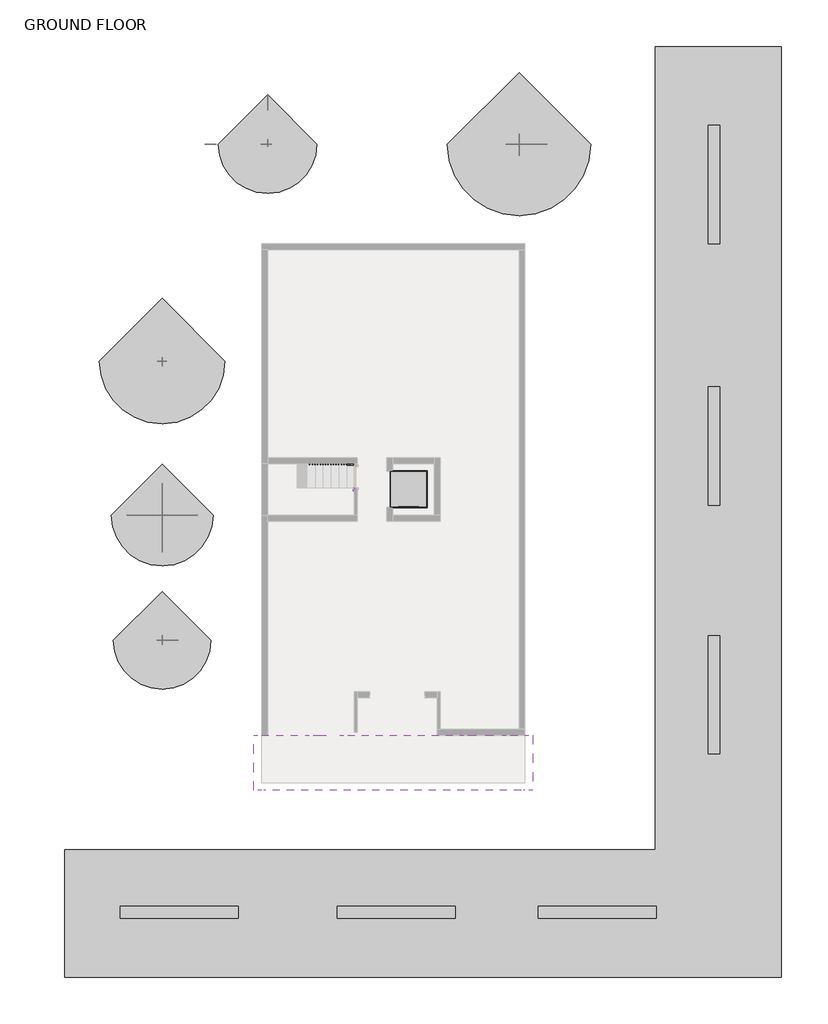
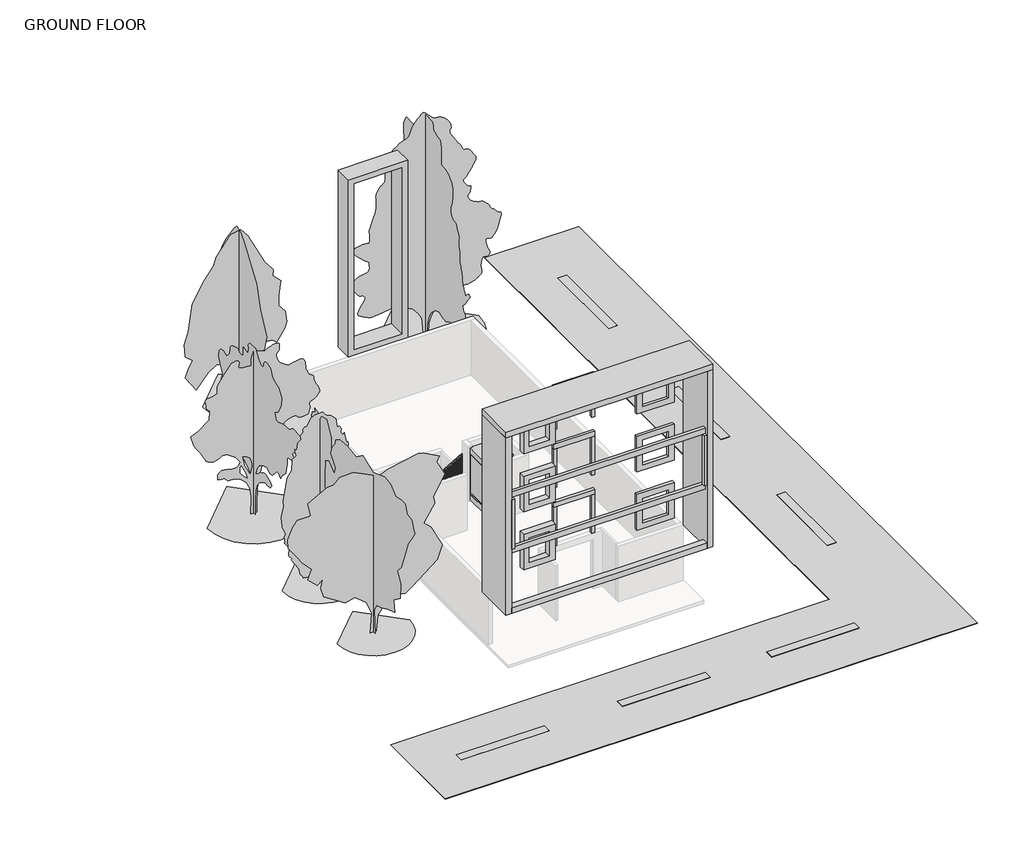
# One storey, part 2 of 2: 5 geographic elements, 3 proxies, 2 railings.
"""IFC4 building model written with IfcOpenShell, lengths in millimetres."""

from ifc_helpers import new_model, si_unit, frame, origin, place, context, project, spatial, polyline, outline, extrude, faceted_brep, transform, mapped, element, save
from components import generic_models_1_generic_models_1_5d1bbf4d, generic_models_2_generic_models_2_e2c80ef7, lift_glass_2_lift_with_hydraulic_ram_a28bd677, rpc_tree_conifer_chinese_juniper_7_2d11b09a, rpc_tree_deciduous_japanese_cherry_15_4daa029f, rpc_tree_fall_lombardy_poplar_40_01077960, rpc_tree_fall_service_berry_25_2_d25f016d, rpc_tree_fall_white_ash_30_ca342e74

model = new_model("IFC4")

# Units and contexts
model_context = context("Model", 3, world=origin())
ifc_project = project(units=[si_unit("LENGTHUNIT", "METRE", prefix="MILLI")], contexts=[model_context])

# Site, building, storey
site = spatial("IfcSite", under=ifc_project)
building = spatial("IfcBuilding", under=site)
storey = spatial("IfcBuildingStorey", under=building, Name="GROUND FLOOR", Elevation=0.0)

# Proxies
placement = place(None, origin())
generic_models_1_generic_models_1_shape = generic_models_1_generic_models_1_5d1bbf4d(model_context)
element("IfcBuildingElementProxy", 1, Name="Generic Models 1 : Generic Models 1", ObjectType="Generic Models 1 : Generic Models 1", at=placement, inside=storey, context=model_context, shape_type="MappedRepresentation", body=[
    mapped(generic_models_1_generic_models_1_shape, transform((0.0, 0.0, 0.0), x_axis=(1.0, 0.0, 0.0), y_axis=(0.0, 1.0, 0.0), z_axis=(0.0, 0.0, 1.0))),
])
generic_models_2_generic_models_2_shape = generic_models_2_generic_models_2_e2c80ef7(model_context)
element("IfcBuildingElementProxy", 2, Name="Generic Models 2 : Generic Models 2", ObjectType="Generic Models 2 : Generic Models 2", at=placement, inside=storey, context=model_context, shape_type="MappedRepresentation", body=[
    mapped(generic_models_2_generic_models_2_shape, transform((0.0, 0.0, 0.0), x_axis=(1.0, 0.0, 0.0), y_axis=(0.0, 1.0, 0.0), z_axis=(0.0, 0.0, 1.0))),
])
lift_glass_2_lift_with_hydraulic_ram_shape = lift_glass_2_lift_with_hydraulic_ram_a28bd677(model_context)
element("IfcBuildingElementProxy", 3, Name="Lift Glass (2) : Lift with Hydraulic Ram", ObjectType="Lift Glass (2) : Lift with Hydraulic Ram", at=placement, inside=storey, context=model_context, shape_type="MappedRepresentation", body=[
    mapped(lift_glass_2_lift_with_hydraulic_ram_shape, transform((-718.3147577, 521.6900134, 381.0), x_axis=(1.0, 0.0, 0.0), y_axis=(0.0, 1.0, 0.0), z_axis=(0.0, 0.0, 1.0))),
])

# Geographic elements
rpc_tree_conifer_chinese_juniper_7_shape = rpc_tree_conifer_chinese_juniper_7_2d11b09a(model_context)
element("IfcGeographicElement", 4, ObjectType="RPC Tree - Conifer : Chinese Juniper - 7'", at=placement, inside=storey, context=model_context, shape_type="MappedRepresentation", body=[
    mapped(rpc_tree_conifer_chinese_juniper_7_shape, transform((-10206.5255752, -431.3846737, -152.4), x_axis=(1.0, 0.0, 0.0), y_axis=(0.0, 1.0, 0.0), z_axis=(0.0, 0.0, 1.0))),
])
rpc_tree_deciduous_japanese_cherry_15_shape = rpc_tree_deciduous_japanese_cherry_15_4daa029f(model_context)
element("IfcGeographicElement", 5, ObjectType="RPC Tree - Deciduous : Japanese Cherry - 15'", at=placement, inside=storey, context=model_context, shape_type="MappedRepresentation", body=[
    mapped(rpc_tree_deciduous_japanese_cherry_15_shape, transform((-10206.3289041, 5524.9153263, -152.4), x_axis=(1.0, 0.0, 0.0), y_axis=(0.0, 1.0, 0.0), z_axis=(0.0, 0.0, 1.0))),
])
rpc_tree_fall_lombardy_poplar_40_shape = rpc_tree_fall_lombardy_poplar_40_01077960(model_context)
element("IfcGeographicElement", 6, ObjectType="RPC Tree - Fall : Lombardy Poplar - 40'", at=placement, inside=storey, context=model_context, shape_type="MappedRepresentation", body=[
    mapped(rpc_tree_fall_lombardy_poplar_40_shape, transform((3585.8710959, 13906.9153263, -152.4), x_axis=(1.0, 0.0, 0.0), y_axis=(0.0, 1.0, 0.0), z_axis=(0.0, 0.0, 1.0))),
])
rpc_tree_fall_service_berry_25_2_shape = rpc_tree_fall_service_berry_25_2_d25f016d(model_context)
element("IfcGeographicElement", 7, ObjectType="RPC Tree - Fall : Service Berry - 25' 2", at=placement, inside=storey, context=model_context, shape_type="MappedRepresentation", body=[
    mapped(rpc_tree_fall_service_berry_25_2_shape, transform((-10206.3289041, -5270.0846737, -152.4), x_axis=(1.0, 0.0, 0.0), y_axis=(0.0, 1.0, 0.0), z_axis=(0.0, 0.0, 1.0))),
])
rpc_tree_fall_white_ash_30_shape = rpc_tree_fall_white_ash_30_ca342e74(model_context)
element("IfcGeographicElement", 8, ObjectType="RPC Tree - Fall : White Ash - 30'", at=placement, inside=storey, context=model_context, shape_type="MappedRepresentation", body=[
    mapped(rpc_tree_fall_white_ash_30_shape, transform((-6129.6289041, 13906.9153263, -152.4), x_axis=(1.0, 0.0, 0.0), y_axis=(0.0, 1.0, 0.0), z_axis=(0.0, 0.0, 1.0))),
])

# Railings
element("IfcRailing", 9, ObjectType="Handrail - Rectangular", at=placement, inside=storey, context=model_context, shape_type="SolidModel", body=[
    faceted_brep([(-2776.8289041, 1499.0153263, 1092.2), (-2776.8289041, 1499.0153263, 1033.3886538), (-2776.8289041, 1549.8153263, 1033.3886538), (-2776.8289041, 1549.8153263, 1092.2), (-5215.2289041, 1499.0153263, 2514.6), (-5228.9626405, 1499.0153263, 2463.8), (-5228.9626405, 1549.8153263, 2463.8), (-5215.2289041, 1549.8153263, 2514.6), (-6078.8289041, 1499.0153263, 2514.6), (-6078.8289041, 1499.0153263, 2463.8), (-6129.6289041, 1549.8153263, 2463.8), (-6129.6289041, 1549.8153263, 2514.6), (-6078.8289041, -380.5846737, 2514.6), (-6078.8289041, -380.5846737, 2463.8), (-6129.6289041, -431.3846737, 2463.8), (-6129.6289041, -431.3846737, 2514.6), (-5520.0289041, -380.5846737, 2514.6), (-5506.2951677, -380.5846737, 2463.8), (-5506.2951677, -431.3846737, 2463.8), (-5520.0289041, -431.3846737, 2514.6), (-2776.8289041, -380.5846737, 4114.8), (-2776.8289041, -431.3846737, 4114.8), (-2776.8289041, -431.3846737, 4055.9886538), (-2776.8289041, -380.5846737, 4055.9886538)], [[[0, 1, 2, 3]], [[1, 0, 4, 5]], [[2, 1, 5, 6]], [[3, 2, 6, 7]], [[0, 3, 7, 4]], [[5, 4, 8, 9]], [[6, 5, 9, 10]], [[7, 6, 10, 11]], [[4, 7, 11, 8]], [[9, 8, 12, 13]], [[10, 9, 13, 14]], [[11, 10, 14, 15]], [[8, 11, 15, 12]], [[13, 12, 16, 17]], [[14, 13, 17, 18]], [[15, 14, 18, 19]], [[12, 15, 19, 16]], [[20, 21, 22, 23]], [[17, 16, 20, 23]], [[18, 17, 23, 22]], [[19, 18, 22, 21]], [[16, 19, 21, 20]]]),
    extrude(outline(polyline([(4017.0949038, -2843.5039041), (4005.9824038, -2862.5539041), (3022.6, -2862.5539041), (3022.6, -2843.5039041), (4017.0949038, -2843.5039041)])), frame((0.0, -415.5096737, 0.0), z_axis=(0.0, 1.0, 0.0), x_axis=(0.0, 0.0, 1.0)), (0.0, 0.0, 1.0), 19.05),
    extrude(outline(polyline([(3957.8282371, -2945.1039041), (3946.7157371, -2964.1539041), (3022.6, -2964.1539041), (3022.6, -2945.1039041), (3957.8282371, -2945.1039041)])), frame((0.0, -415.5096737, 0.0), z_axis=(0.0, 1.0, 0.0), x_axis=(0.0, 0.0, 1.0)), (0.0, 0.0, 1.0), 19.05),
    extrude(outline(polyline([(3898.5615704, -3046.7039041), (3887.4490704, -3065.7539041), (3022.6, -3065.7539041), (3022.6, -3046.7039041), (3898.5615704, -3046.7039041)])), frame((0.0, -415.5096737, 0.0), z_axis=(0.0, 1.0, 0.0), x_axis=(0.0, 0.0, 1.0)), (0.0, 0.0, 1.0), 19.05),
    extrude(outline(polyline([(3839.2949038, -3148.3039041), (3828.1824038, -3167.3539041), (2844.8, -3167.3539041), (2844.8, -3148.3039041), (3839.2949038, -3148.3039041)])), frame((0.0, -415.5096737, 0.0), z_axis=(0.0, 1.0, 0.0), x_axis=(0.0, 0.0, 1.0)), (0.0, 0.0, 1.0), 19.05),
    extrude(outline(polyline([(3780.0282371, -3249.9039041), (3768.9157371, -3268.9539041), (2844.8, -3268.9539041), (2844.8, -3249.9039041), (3780.0282371, -3249.9039041)])), frame((0.0, -415.5096737, 0.0), z_axis=(0.0, 1.0, 0.0), x_axis=(0.0, 0.0, 1.0)), (0.0, 0.0, 1.0), 19.05),
    extrude(outline(polyline([(3720.7615704, -3351.5039041), (3709.6490704, -3370.5539041), (2844.8, -3370.5539041), (2844.8, -3351.5039041), (3720.7615704, -3351.5039041)])), frame((0.0, -415.5096737, 0.0), z_axis=(0.0, 1.0, 0.0), x_axis=(0.0, 0.0, 1.0)), (0.0, 0.0, 1.0), 19.05),
    extrude(outline(polyline([(3661.4949038, -3453.1039041), (3650.3824038, -3472.1539041), (2667.0, -3472.1539041), (2667.0, -3453.1039041), (3661.4949038, -3453.1039041)])), frame((0.0, -415.5096737, 0.0), z_axis=(0.0, 1.0, 0.0), x_axis=(0.0, 0.0, 1.0)), (0.0, 0.0, 1.0), 19.05),
    extrude(outline(polyline([(3602.2282371, -3554.7039041), (3591.1157371, -3573.7539041), (2667.0, -3573.7539041), (2667.0, -3554.7039041), (3602.2282371, -3554.7039041)])), frame((0.0, -415.5096737, 0.0), z_axis=(0.0, 1.0, 0.0), x_axis=(0.0, 0.0, 1.0)), (0.0, 0.0, 1.0), 19.05),
    extrude(outline(polyline([(3542.9615704, -3656.3039041), (3531.8490704, -3675.3539041), (2667.0, -3675.3539041), (2667.0, -3656.3039041), (3542.9615704, -3656.3039041)])), frame((0.0, -415.5096737, 0.0), z_axis=(0.0, 1.0, 0.0), x_axis=(0.0, 0.0, 1.0)), (0.0, 0.0, 1.0), 19.05),
    extrude(outline(polyline([(3483.6949038, -3757.9039041), (3472.5824038, -3776.9539041), (2489.2, -3776.9539041), (2489.2, -3757.9039041), (3483.6949038, -3757.9039041)])), frame((0.0, -415.5096737, 0.0), z_axis=(0.0, 1.0, 0.0), x_axis=(0.0, 0.0, 1.0)), (0.0, 0.0, 1.0), 19.05),
    extrude(outline(polyline([(3424.4282371, -3859.5039041), (3413.3157371, -3878.5539041), (2489.2, -3878.5539041), (2489.2, -3859.5039041), (3424.4282371, -3859.5039041)])), frame((0.0, -415.5096737, 0.0), z_axis=(0.0, 1.0, 0.0), x_axis=(0.0, 0.0, 1.0)), (0.0, 0.0, 1.0), 19.05),
    extrude(outline(polyline([(3365.1615704, -3961.1039041), (3354.0490704, -3980.1539041), (2489.2, -3980.1539041), (2489.2, -3961.1039041), (3365.1615704, -3961.1039041)])), frame((0.0, -415.5096737, 0.0), z_axis=(0.0, 1.0, 0.0), x_axis=(0.0, 0.0, 1.0)), (0.0, 0.0, 1.0), 19.05),
    extrude(outline(polyline([(3305.8949038, -4062.7039041), (3294.7824038, -4081.7539041), (2311.4, -4081.7539041), (2311.4, -4062.7039041), (3305.8949038, -4062.7039041)])), frame((0.0, -415.5096737, 0.0), z_axis=(0.0, 1.0, 0.0), x_axis=(0.0, 0.0, 1.0)), (0.0, 0.0, 1.0), 19.05),
    extrude(outline(polyline([(3246.6282371, -4164.3039041), (3235.5157371, -4183.3539041), (2311.4, -4183.3539041), (2311.4, -4164.3039041), (3246.6282371, -4164.3039041)])), frame((0.0, -415.5096737, 0.0), z_axis=(0.0, 1.0, 0.0), x_axis=(0.0, 0.0, 1.0)), (0.0, 0.0, 1.0), 19.05),
    extrude(outline(polyline([(3187.3615704, -4265.9039041), (3176.2490704, -4284.9539041), (2311.4, -4284.9539041), (2311.4, -4265.9039041), (3187.3615704, -4265.9039041)])), frame((0.0, -415.5096737, 0.0), z_axis=(0.0, 1.0, 0.0), x_axis=(0.0, 0.0, 1.0)), (0.0, 0.0, 1.0), 19.05),
    extrude(outline(polyline([(3128.0949038, -4367.5039041), (3116.9824038, -4386.5539041), (2133.6, -4386.5539041), (2133.6, -4367.5039041), (3128.0949038, -4367.5039041)])), frame((0.0, -415.5096737, 0.0), z_axis=(0.0, 1.0, 0.0), x_axis=(0.0, 0.0, 1.0)), (0.0, 0.0, 1.0), 19.05),
    extrude(outline(polyline([(3068.8282371, -4469.1039041), (3057.7157371, -4488.1539041), (2133.6, -4488.1539041), (2133.6, -4469.1039041), (3068.8282371, -4469.1039041)])), frame((0.0, -415.5096737, 0.0), z_axis=(0.0, 1.0, 0.0), x_axis=(0.0, 0.0, 1.0)), (0.0, 0.0, 1.0), 19.05),
    extrude(outline(polyline([(3009.5615704, -4570.7039041), (2998.4490704, -4589.7539041), (2133.6, -4589.7539041), (2133.6, -4570.7039041), (3009.5615704, -4570.7039041)])), frame((0.0, -415.5096737, 0.0), z_axis=(0.0, 1.0, 0.0), x_axis=(0.0, 0.0, 1.0)), (0.0, 0.0, 1.0), 19.05),
    extrude(outline(polyline([(2950.2949038, -4672.3039041), (2939.1824038, -4691.3539041), (1955.8, -4691.3539041), (1955.8, -4672.3039041), (2950.2949038, -4672.3039041)])), frame((0.0, -415.5096737, 0.0), z_axis=(0.0, 1.0, 0.0), x_axis=(0.0, 0.0, 1.0)), (0.0, 0.0, 1.0), 19.05),
    extrude(outline(polyline([(2891.0282371, -4773.9039041), (2879.9157371, -4792.9539041), (1955.8, -4792.9539041), (1955.8, -4773.9039041), (2891.0282371, -4773.9039041)])), frame((0.0, -415.5096737, 0.0), z_axis=(0.0, 1.0, 0.0), x_axis=(0.0, 0.0, 1.0)), (0.0, 0.0, 1.0), 19.05),
    extrude(outline(polyline([(2831.7615704, -4875.5039041), (2820.6490704, -4894.5539041), (1955.8, -4894.5539041), (1955.8, -4875.5039041), (2831.7615704, -4875.5039041)])), frame((0.0, -415.5096737, 0.0), z_axis=(0.0, 1.0, 0.0), x_axis=(0.0, 0.0, 1.0)), (0.0, 0.0, 1.0), 19.05),
    extrude(outline(polyline([(2772.4949038, -4977.1039041), (2761.3824038, -4996.1539041), (1778.0, -4996.1539041), (1778.0, -4977.1039041), (2772.4949038, -4977.1039041)])), frame((0.0, -415.5096737, 0.0), z_axis=(0.0, 1.0, 0.0), x_axis=(0.0, 0.0, 1.0)), (0.0, 0.0, 1.0), 19.05),
    extrude(outline(polyline([(2713.2282371, -5078.7039041), (2702.1157371, -5097.7539041), (1778.0, -5097.7539041), (1778.0, -5078.7039041), (2713.2282371, -5078.7039041)])), frame((0.0, -415.5096737, 0.0), z_axis=(0.0, 1.0, 0.0), x_axis=(0.0, 0.0, 1.0)), (0.0, 0.0, 1.0), 19.05),
    extrude(outline(polyline([(2653.9615704, -5180.3039041), (2642.8490704, -5199.3539041), (1778.0, -5199.3539041), (1778.0, -5180.3039041), (2653.9615704, -5180.3039041)])), frame((0.0, -415.5096737, 0.0), z_axis=(0.0, 1.0, 0.0), x_axis=(0.0, 0.0, 1.0)), (0.0, 0.0, 1.0), 19.05),
    extrude(outline(polyline([(2594.6949038, -5281.9039041), (2583.5824038, -5300.9539041), (1600.2, -5300.9539041), (1600.2, -5281.9039041), (2594.6949038, -5281.9039041)])), frame((0.0, -415.5096737, 0.0), z_axis=(0.0, 1.0, 0.0), x_axis=(0.0, 0.0, 1.0)), (0.0, 0.0, 1.0), 19.05),
    extrude(outline(polyline([(2535.4282371, -5383.5039041), (2524.3157371, -5402.5539041), (1600.2, -5402.5539041), (1600.2, -5383.5039041), (2535.4282371, -5383.5039041)])), frame((0.0, -415.5096737, 0.0), z_axis=(0.0, 1.0, 0.0), x_axis=(0.0, 0.0, 1.0)), (0.0, 0.0, 1.0), 19.05),
    extrude(outline(polyline([(2476.1615704, -5485.1039041), (2465.0490704, -5504.1539041), (1600.2, -5504.1539041), (1600.2, -5485.1039041), (2476.1615704, -5485.1039041)])), frame((0.0, -415.5096737, 0.0), z_axis=(0.0, 1.0, 0.0), x_axis=(0.0, 0.0, 1.0)), (0.0, 0.0, 1.0), 19.05),
    extrude(outline(polyline([(-5605.7539041, -415.5096737), (-5605.7539041, -396.4596737), (-5586.7039041, -396.4596737), (-5586.7039041, -415.5096737), (-5605.7539041, -415.5096737)])), frame((0.0, 0.0, 1600.2), z_axis=(0.0, 0.0, 1.0), x_axis=(1.0, 0.0, 0.0)), (0.0, 0.0, 1.0), 863.6),
    extrude(outline(polyline([(-5707.3539041, -415.5096737), (-5707.3539041, -396.4596737), (-5688.3039041, -396.4596737), (-5688.3039041, -415.5096737), (-5707.3539041, -415.5096737)])), frame((0.0, 0.0, 1600.2), z_axis=(0.0, 0.0, 1.0), x_axis=(1.0, 0.0, 0.0)), (0.0, 0.0, 1.0), 863.6),
    extrude(outline(polyline([(-5808.9539041, -415.5096737), (-5808.9539041, -396.4596737), (-5789.9039041, -396.4596737), (-5789.9039041, -415.5096737), (-5808.9539041, -415.5096737)])), frame((0.0, 0.0, 1600.2), z_axis=(0.0, 0.0, 1.0), x_axis=(1.0, 0.0, 0.0)), (0.0, 0.0, 1.0), 863.6),
    extrude(outline(polyline([(-5910.5539041, -415.5096737), (-5910.5539041, -396.4596737), (-5891.5039041, -396.4596737), (-5891.5039041, -415.5096737), (-5910.5539041, -415.5096737)])), frame((0.0, 0.0, 1600.2), z_axis=(0.0, 0.0, 1.0), x_axis=(1.0, 0.0, 0.0)), (0.0, 0.0, 1.0), 863.6),
    extrude(outline(polyline([(-6012.1539041, -415.5096737), (-6012.1539041, -396.4596737), (-5993.1039041, -396.4596737), (-5993.1039041, -415.5096737), (-6012.1539041, -415.5096737)])), frame((0.0, 0.0, 1600.2), z_axis=(0.0, 0.0, 1.0), x_axis=(1.0, 0.0, 0.0)), (0.0, 0.0, 1.0), 863.6),
    extrude(outline(polyline([(-6113.7539041, -294.8596737), (-6094.7039041, -294.8596737), (-6094.7039041, -313.9096737), (-6113.7539041, -313.9096737), (-6113.7539041, -294.8596737)])), frame((0.0, 0.0, 1600.2), z_axis=(0.0, 0.0, 1.0), x_axis=(1.0, 0.0, 0.0)), (0.0, 0.0, 1.0), 863.6),
    extrude(outline(polyline([(-6113.7539041, -193.2596737), (-6094.7039041, -193.2596737), (-6094.7039041, -212.3096737), (-6113.7539041, -212.3096737), (-6113.7539041, -193.2596737)])), frame((0.0, 0.0, 1600.2), z_axis=(0.0, 0.0, 1.0), x_axis=(1.0, 0.0, 0.0)), (0.0, 0.0, 1.0), 863.6),
    extrude(outline(polyline([(-6113.7539041, -91.6596737), (-6094.7039041, -91.6596737), (-6094.7039041, -110.7096737), (-6113.7539041, -110.7096737), (-6113.7539041, -91.6596737)])), frame((0.0, 0.0, 1600.2), z_axis=(0.0, 0.0, 1.0), x_axis=(1.0, 0.0, 0.0)), (0.0, 0.0, 1.0), 863.6),
    extrude(outline(polyline([(-6113.7539041, 9.9403263), (-6094.7039041, 9.9403263), (-6094.7039041, -9.1096737), (-6113.7539041, -9.1096737), (-6113.7539041, 9.9403263)])), frame((0.0, 0.0, 1600.2), z_axis=(0.0, 0.0, 1.0), x_axis=(1.0, 0.0, 0.0)), (0.0, 0.0, 1.0), 863.6),
    extrude(outline(polyline([(-6113.7539041, 111.5403263), (-6094.7039041, 111.5403263), (-6094.7039041, 92.4903263), (-6113.7539041, 92.4903263), (-6113.7539041, 111.5403263)])), frame((0.0, 0.0, 1600.2), z_axis=(0.0, 0.0, 1.0), x_axis=(1.0, 0.0, 0.0)), (0.0, 0.0, 1.0), 863.6),
    extrude(outline(polyline([(-6113.7539041, 213.1403263), (-6094.7039041, 213.1403263), (-6094.7039041, 194.0903263), (-6113.7539041, 194.0903263), (-6113.7539041, 213.1403263)])), frame((0.0, 0.0, 1600.2), z_axis=(0.0, 0.0, 1.0), x_axis=(1.0, 0.0, 0.0)), (0.0, 0.0, 1.0), 863.6),
    extrude(outline(polyline([(-6113.7539041, 314.7403263), (-6094.7039041, 314.7403263), (-6094.7039041, 295.6903263), (-6113.7539041, 295.6903263), (-6113.7539041, 314.7403263)])), frame((0.0, 0.0, 1600.2), z_axis=(0.0, 0.0, 1.0), x_axis=(1.0, 0.0, 0.0)), (0.0, 0.0, 1.0), 863.6),
    extrude(outline(polyline([(-6113.7539041, 416.3403263), (-6094.7039041, 416.3403263), (-6094.7039041, 397.2903263), (-6113.7539041, 397.2903263), (-6113.7539041, 416.3403263)])), frame((0.0, 0.0, 1600.2), z_axis=(0.0, 0.0, 1.0), x_axis=(1.0, 0.0, 0.0)), (0.0, 0.0, 1.0), 863.6),
    extrude(outline(polyline([(-6113.7539041, 517.9403263), (-6094.7039041, 517.9403263), (-6094.7039041, 498.8903263), (-6113.7539041, 498.8903263), (-6113.7539041, 517.9403263)])), frame((0.0, 0.0, 1600.2), z_axis=(0.0, 0.0, 1.0), x_axis=(1.0, 0.0, 0.0)), (0.0, 0.0, 1.0), 863.6),
    extrude(outline(polyline([(-6113.7539041, 619.5403263), (-6094.7039041, 619.5403263), (-6094.7039041, 600.4903263), (-6113.7539041, 600.4903263), (-6113.7539041, 619.5403263)])), frame((0.0, 0.0, 1600.2), z_axis=(0.0, 0.0, 1.0), x_axis=(1.0, 0.0, 0.0)), (0.0, 0.0, 1.0), 863.6),
    extrude(outline(polyline([(-6113.7539041, 721.1403263), (-6094.7039041, 721.1403263), (-6094.7039041, 702.0903263), (-6113.7539041, 702.0903263), (-6113.7539041, 721.1403263)])), frame((0.0, 0.0, 1600.2), z_axis=(0.0, 0.0, 1.0), x_axis=(1.0, 0.0, 0.0)), (0.0, 0.0, 1.0), 863.6),
    extrude(outline(polyline([(-6113.7539041, 822.7403263), (-6094.7039041, 822.7403263), (-6094.7039041, 803.6903263), (-6113.7539041, 803.6903263), (-6113.7539041, 822.7403263)])), frame((0.0, 0.0, 1600.2), z_axis=(0.0, 0.0, 1.0), x_axis=(1.0, 0.0, 0.0)), (0.0, 0.0, 1.0), 863.6),
    extrude(outline(polyline([(-6113.7539041, 924.3403263), (-6094.7039041, 924.3403263), (-6094.7039041, 905.2903263), (-6113.7539041, 905.2903263), (-6113.7539041, 924.3403263)])), frame((0.0, 0.0, 1600.2), z_axis=(0.0, 0.0, 1.0), x_axis=(1.0, 0.0, 0.0)), (0.0, 0.0, 1.0), 863.6),
    extrude(outline(polyline([(-6113.7539041, 1025.9403263), (-6094.7039041, 1025.9403263), (-6094.7039041, 1006.8903263), (-6113.7539041, 1006.8903263), (-6113.7539041, 1025.9403263)])), frame((0.0, 0.0, 1600.2), z_axis=(0.0, 0.0, 1.0), x_axis=(1.0, 0.0, 0.0)), (0.0, 0.0, 1.0), 863.6),
    extrude(outline(polyline([(-6113.7539041, 1127.5403263), (-6094.7039041, 1127.5403263), (-6094.7039041, 1108.4903263), (-6113.7539041, 1108.4903263), (-6113.7539041, 1127.5403263)])), frame((0.0, 0.0, 1600.2), z_axis=(0.0, 0.0, 1.0), x_axis=(1.0, 0.0, 0.0)), (0.0, 0.0, 1.0), 863.6),
    extrude(outline(polyline([(-6113.7539041, 1229.1403263), (-6094.7039041, 1229.1403263), (-6094.7039041, 1210.0903263), (-6113.7539041, 1210.0903263), (-6113.7539041, 1229.1403263)])), frame((0.0, 0.0, 1600.2), z_axis=(0.0, 0.0, 1.0), x_axis=(1.0, 0.0, 0.0)), (0.0, 0.0, 1.0), 863.6),
    extrude(outline(polyline([(-6113.7539041, 1330.7403263), (-6094.7039041, 1330.7403263), (-6094.7039041, 1311.6903263), (-6113.7539041, 1311.6903263), (-6113.7539041, 1330.7403263)])), frame((0.0, 0.0, 1600.2), z_axis=(0.0, 0.0, 1.0), x_axis=(1.0, 0.0, 0.0)), (0.0, 0.0, 1.0), 863.6),
    extrude(outline(polyline([(-6113.7539041, 1432.3403263), (-6094.7039041, 1432.3403263), (-6094.7039041, 1413.2903263), (-6113.7539041, 1413.2903263), (-6113.7539041, 1432.3403263)])), frame((0.0, 0.0, 1600.2), z_axis=(0.0, 0.0, 1.0), x_axis=(1.0, 0.0, 0.0)), (0.0, 0.0, 1.0), 863.6),
    extrude(outline(polyline([(-6018.5039041, 1533.9403263), (-6018.5039041, 1514.8903263), (-6037.5539041, 1514.8903263), (-6037.5539041, 1533.9403263), (-6018.5039041, 1533.9403263)])), frame((0.0, 0.0, 1600.2), z_axis=(0.0, 0.0, 1.0), x_axis=(1.0, 0.0, 0.0)), (0.0, 0.0, 1.0), 863.6),
    extrude(outline(polyline([(-5916.9039041, 1533.9403263), (-5916.9039041, 1514.8903263), (-5935.9539041, 1514.8903263), (-5935.9539041, 1533.9403263), (-5916.9039041, 1533.9403263)])), frame((0.0, 0.0, 1600.2), z_axis=(0.0, 0.0, 1.0), x_axis=(1.0, 0.0, 0.0)), (0.0, 0.0, 1.0), 863.6),
    extrude(outline(polyline([(-5815.3039041, 1533.9403263), (-5815.3039041, 1514.8903263), (-5834.3539041, 1514.8903263), (-5834.3539041, 1533.9403263), (-5815.3039041, 1533.9403263)])), frame((0.0, 0.0, 1600.2), z_axis=(0.0, 0.0, 1.0), x_axis=(1.0, 0.0, 0.0)), (0.0, 0.0, 1.0), 863.6),
    extrude(outline(polyline([(-5713.7039041, 1533.9403263), (-5713.7039041, 1514.8903263), (-5732.7539041, 1514.8903263), (-5732.7539041, 1533.9403263), (-5713.7039041, 1533.9403263)])), frame((0.0, 0.0, 1600.2), z_axis=(0.0, 0.0, 1.0), x_axis=(1.0, 0.0, 0.0)), (0.0, 0.0, 1.0), 863.6),
    extrude(outline(polyline([(-5612.1039041, 1533.9403263), (-5612.1039041, 1514.8903263), (-5631.1539041, 1514.8903263), (-5631.1539041, 1533.9403263), (-5612.1039041, 1533.9403263)])), frame((0.0, 0.0, 1600.2), z_axis=(0.0, 0.0, 1.0), x_axis=(1.0, 0.0, 0.0)), (0.0, 0.0, 1.0), 863.6),
    extrude(outline(polyline([(-5510.5039041, 1533.9403263), (-5510.5039041, 1514.8903263), (-5529.5539041, 1514.8903263), (-5529.5539041, 1533.9403263), (-5510.5039041, 1533.9403263)])), frame((0.0, 0.0, 1600.2), z_axis=(0.0, 0.0, 1.0), x_axis=(1.0, 0.0, 0.0)), (0.0, 0.0, 1.0), 863.6),
    extrude(outline(polyline([(-5408.9039041, 1533.9403263), (-5408.9039041, 1514.8903263), (-5427.9539041, 1514.8903263), (-5427.9539041, 1533.9403263), (-5408.9039041, 1533.9403263)])), frame((0.0, 0.0, 1600.2), z_axis=(0.0, 0.0, 1.0), x_axis=(1.0, 0.0, 0.0)), (0.0, 0.0, 1.0), 863.6),
    extrude(outline(polyline([(-5307.3039041, 1533.9403263), (-5307.3039041, 1514.8903263), (-5326.3539041, 1514.8903263), (-5326.3539041, 1533.9403263), (-5307.3039041, 1533.9403263)])), frame((0.0, 0.0, 1600.2), z_axis=(0.0, 0.0, 1.0), x_axis=(1.0, 0.0, 0.0)), (0.0, 0.0, 1.0), 863.6),
    extrude(outline(polyline([(2450.2324038, -5205.7039041), (2461.3449038, -5224.7539041), (1600.2, -5224.7539041), (1600.2, -5205.7039041), (2450.2324038, -5205.7039041)])), frame((0.0, 1514.8903263, 0.0), z_axis=(0.0, 1.0, 0.0), x_axis=(0.0, 0.0, 1.0)), (0.0, 0.0, 1.0), 19.05),
    extrude(outline(polyline([(2390.9657371, -5104.1039041), (2402.0782371, -5123.1539041), (1422.4, -5123.1539041), (1422.4, -5104.1039041), (2390.9657371, -5104.1039041)])), frame((0.0, 1514.8903263, 0.0), z_axis=(0.0, 1.0, 0.0), x_axis=(0.0, 0.0, 1.0)), (0.0, 0.0, 1.0), 19.05),
    extrude(outline(polyline([(2331.6990704, -5002.5039041), (2342.8115704, -5021.5539041), (1422.4, -5021.5539041), (1422.4, -5002.5039041), (2331.6990704, -5002.5039041)])), frame((0.0, 1514.8903263, 0.0), z_axis=(0.0, 1.0, 0.0), x_axis=(0.0, 0.0, 1.0)), (0.0, 0.0, 1.0), 19.05),
    extrude(outline(polyline([(2272.4324038, -4900.9039041), (2283.5449038, -4919.9539041), (1422.4, -4919.9539041), (1422.4, -4900.9039041), (2272.4324038, -4900.9039041)])), frame((0.0, 1514.8903263, 0.0), z_axis=(0.0, 1.0, 0.0), x_axis=(0.0, 0.0, 1.0)), (0.0, 0.0, 1.0), 19.05),
    extrude(outline(polyline([(2213.1657371, -4799.3039041), (2224.2782371, -4818.3539041), (1244.6, -4818.3539041), (1244.6, -4799.3039041), (2213.1657371, -4799.3039041)])), frame((0.0, 1514.8903263, 0.0), z_axis=(0.0, 1.0, 0.0), x_axis=(0.0, 0.0, 1.0)), (0.0, 0.0, 1.0), 19.05),
    extrude(outline(polyline([(2153.8990704, -4697.7039041), (2165.0115704, -4716.7539041), (1244.6, -4716.7539041), (1244.6, -4697.7039041), (2153.8990704, -4697.7039041)])), frame((0.0, 1514.8903263, 0.0), z_axis=(0.0, 1.0, 0.0), x_axis=(0.0, 0.0, 1.0)), (0.0, 0.0, 1.0), 19.05),
    extrude(outline(polyline([(2094.6324038, -4596.1039041), (2105.7449038, -4615.1539041), (1244.6, -4615.1539041), (1244.6, -4596.1039041), (2094.6324038, -4596.1039041)])), frame((0.0, 1514.8903263, 0.0), z_axis=(0.0, 1.0, 0.0), x_axis=(0.0, 0.0, 1.0)), (0.0, 0.0, 1.0), 19.05),
    extrude(outline(polyline([(2035.3657371, -4494.5039041), (2046.4782371, -4513.5539041), (1066.8, -4513.5539041), (1066.8, -4494.5039041), (2035.3657371, -4494.5039041)])), frame((0.0, 1514.8903263, 0.0), z_axis=(0.0, 1.0, 0.0), x_axis=(0.0, 0.0, 1.0)), (0.0, 0.0, 1.0), 19.05),
    extrude(outline(polyline([(1976.0990704, -4392.9039041), (1987.2115704, -4411.9539041), (1066.8, -4411.9539041), (1066.8, -4392.9039041), (1976.0990704, -4392.9039041)])), frame((0.0, 1514.8903263, 0.0), z_axis=(0.0, 1.0, 0.0), x_axis=(0.0, 0.0, 1.0)), (0.0, 0.0, 1.0), 19.05),
    extrude(outline(polyline([(1916.8324038, -4291.3039041), (1927.9449038, -4310.3539041), (1066.8, -4310.3539041), (1066.8, -4291.3039041), (1916.8324038, -4291.3039041)])), frame((0.0, 1514.8903263, 0.0), z_axis=(0.0, 1.0, 0.0), x_axis=(0.0, 0.0, 1.0)), (0.0, 0.0, 1.0), 19.05),
    extrude(outline(polyline([(1857.5657371, -4189.7039041), (1868.6782371, -4208.7539041), (889.0, -4208.7539041), (889.0, -4189.7039041), (1857.5657371, -4189.7039041)])), frame((0.0, 1514.8903263, 0.0), z_axis=(0.0, 1.0, 0.0), x_axis=(0.0, 0.0, 1.0)), (0.0, 0.0, 1.0), 19.05),
    extrude(outline(polyline([(1798.2990704, -4088.1039041), (1809.4115704, -4107.1539041), (889.0, -4107.1539041), (889.0, -4088.1039041), (1798.2990704, -4088.1039041)])), frame((0.0, 1514.8903263, 0.0), z_axis=(0.0, 1.0, 0.0), x_axis=(0.0, 0.0, 1.0)), (0.0, 0.0, 1.0), 19.05),
    extrude(outline(polyline([(1739.0324038, -3986.5039041), (1750.1449038, -4005.5539041), (889.0, -4005.5539041), (889.0, -3986.5039041), (1739.0324038, -3986.5039041)])), frame((0.0, 1514.8903263, 0.0), z_axis=(0.0, 1.0, 0.0), x_axis=(0.0, 0.0, 1.0)), (0.0, 0.0, 1.0), 19.05),
    extrude(outline(polyline([(1679.7657371, -3884.9039041), (1690.8782371, -3903.9539041), (711.2, -3903.9539041), (711.2, -3884.9039041), (1679.7657371, -3884.9039041)])), frame((0.0, 1514.8903263, 0.0), z_axis=(0.0, 1.0, 0.0), x_axis=(0.0, 0.0, 1.0)), (0.0, 0.0, 1.0), 19.05),
    extrude(outline(polyline([(1620.4990704, -3783.3039041), (1631.6115704, -3802.3539041), (711.2, -3802.3539041), (711.2, -3783.3039041), (1620.4990704, -3783.3039041)])), frame((0.0, 1514.8903263, 0.0), z_axis=(0.0, 1.0, 0.0), x_axis=(0.0, 0.0, 1.0)), (0.0, 0.0, 1.0), 19.05),
    extrude(outline(polyline([(1561.2324038, -3681.7039041), (1572.3449038, -3700.7539041), (711.2, -3700.7539041), (711.2, -3681.7039041), (1561.2324038, -3681.7039041)])), frame((0.0, 1514.8903263, 0.0), z_axis=(0.0, 1.0, 0.0), x_axis=(0.0, 0.0, 1.0)), (0.0, 0.0, 1.0), 19.05),
    extrude(outline(polyline([(1501.9657371, -3580.1039041), (1513.0782371, -3599.1539041), (533.4, -3599.1539041), (533.4, -3580.1039041), (1501.9657371, -3580.1039041)])), frame((0.0, 1514.8903263, 0.0), z_axis=(0.0, 1.0, 0.0), x_axis=(0.0, 0.0, 1.0)), (0.0, 0.0, 1.0), 19.05),
    extrude(outline(polyline([(1442.6990704, -3478.5039041), (1453.8115704, -3497.5539041), (533.4, -3497.5539041), (533.4, -3478.5039041), (1442.6990704, -3478.5039041)])), frame((0.0, 1514.8903263, 0.0), z_axis=(0.0, 1.0, 0.0), x_axis=(0.0, 0.0, 1.0)), (0.0, 0.0, 1.0), 19.05),
    extrude(outline(polyline([(1383.4324038, -3376.9039041), (1394.5449038, -3395.9539041), (533.4, -3395.9539041), (533.4, -3376.9039041), (1383.4324038, -3376.9039041)])), frame((0.0, 1514.8903263, 0.0), z_axis=(0.0, 1.0, 0.0), x_axis=(0.0, 0.0, 1.0)), (0.0, 0.0, 1.0), 19.05),
    extrude(outline(polyline([(1324.1657371, -3275.3039041), (1335.2782371, -3294.3539041), (355.6, -3294.3539041), (355.6, -3275.3039041), (1324.1657371, -3275.3039041)])), frame((0.0, 1514.8903263, 0.0), z_axis=(0.0, 1.0, 0.0), x_axis=(0.0, 0.0, 1.0)), (0.0, 0.0, 1.0), 19.05),
    extrude(outline(polyline([(1264.8990704, -3173.7039041), (1276.0115704, -3192.7539041), (355.6, -3192.7539041), (355.6, -3173.7039041), (1264.8990704, -3173.7039041)])), frame((0.0, 1514.8903263, 0.0), z_axis=(0.0, 1.0, 0.0), x_axis=(0.0, 0.0, 1.0)), (0.0, 0.0, 1.0), 19.05),
    extrude(outline(polyline([(1205.6324038, -3072.1039041), (1216.7449038, -3091.1539041), (355.6, -3091.1539041), (355.6, -3072.1039041), (1205.6324038, -3072.1039041)])), frame((0.0, 1514.8903263, 0.0), z_axis=(0.0, 1.0, 0.0), x_axis=(0.0, 0.0, 1.0)), (0.0, 0.0, 1.0), 19.05),
    extrude(outline(polyline([(1146.3657371, -2970.5039041), (1157.4782371, -2989.5539041), (177.8, -2989.5539041), (177.8, -2970.5039041), (1146.3657371, -2970.5039041)])), frame((0.0, 1514.8903263, 0.0), z_axis=(0.0, 1.0, 0.0), x_axis=(0.0, 0.0, 1.0)), (0.0, 0.0, 1.0), 19.05),
    extrude(outline(polyline([(1087.0990704, -2868.9039041), (1098.2115704, -2887.9539041), (177.8, -2887.9539041), (177.8, -2868.9039041), (1087.0990704, -2868.9039041)])), frame((0.0, 1514.8903263, 0.0), z_axis=(0.0, 1.0, 0.0), x_axis=(0.0, 0.0, 1.0)), (0.0, 0.0, 1.0), 19.05),
    extrude(outline(polyline([(-6113.7539041, -396.4596737), (-6094.7039041, -396.4596737), (-6094.7039041, -415.5096737), (-6113.7539041, -415.5096737), (-6113.7539041, -396.4596737)])), frame((0.0, 0.0, 1600.2), z_axis=(0.0, 0.0, 1.0), x_axis=(1.0, 0.0, 0.0)), (0.0, 0.0, 1.0), 863.6),
    extrude(outline(polyline([(-6094.7039041, 1533.9403263), (-6094.7039041, 1514.8903263), (-6113.7539041, 1514.8903263), (-6113.7539041, 1533.9403263), (-6094.7039041, 1533.9403263)])), frame((0.0, 0.0, 1600.2), z_axis=(0.0, 0.0, 1.0), x_axis=(1.0, 0.0, 0.0)), (0.0, 0.0, 1.0), 863.6),
    extrude(outline(polyline([(4055.9886538, -2776.8289041), (4044.8761538, -2795.8789041), (3022.6, -2795.8789041), (3022.6, -2776.8289041), (4055.9886538, -2776.8289041)])), frame((0.0, -415.5096737, 0.0), z_axis=(0.0, 1.0, 0.0), x_axis=(0.0, 0.0, 1.0)), (0.0, 0.0, 1.0), 19.05),
    extrude(outline(polyline([(1033.3886538, -2776.8289041), (1044.5011538, -2795.8789041), (177.8, -2795.8789041), (177.8, -2776.8289041), (1033.3886538, -2776.8289041)])), frame((0.0, 1514.8903263, 0.0), z_axis=(0.0, 1.0, 0.0), x_axis=(0.0, 0.0, 1.0)), (0.0, 0.0, 1.0), 19.05),
])
element("IfcRailing", 10, ObjectType="Handrail - Rectangular", at=placement, inside=storey, context=model_context, shape_type="SweptSolid", body=[
    extrude(outline(polyline([(-2827.6289041, 635.4153263), (-2776.8289041, 635.4153263), (-2776.8289041, 483.0153263), (-2827.6289041, 483.0153263), (-2827.6289041, 635.4153263)])), frame((0.0, 0.0, 2463.8), z_axis=(0.0, 0.0, 1.0), x_axis=(1.0, 0.0, 0.0)), (0.0, 0.0, 1.0), 50.8),
    extrude(outline(polyline([(-2792.7039041, 543.3403263), (-2792.7039041, 524.2903263), (-2811.7539041, 524.2903263), (-2811.7539041, 543.3403263), (-2792.7039041, 543.3403263)])), frame((0.0, 0.0, 1600.2), z_axis=(0.0, 0.0, 1.0), x_axis=(1.0, 0.0, 0.0)), (0.0, 0.0, 1.0), 863.6),
    extrude(outline(polyline([(-2792.7039041, 502.0653263), (-2792.7039041, 483.0153263), (-2811.7539041, 483.0153263), (-2811.7539041, 502.0653263), (-2792.7039041, 502.0653263)])), frame((0.0, 0.0, 1600.2), z_axis=(0.0, 0.0, 1.0), x_axis=(1.0, 0.0, 0.0)), (0.0, 0.0, 1.0), 863.6),
    extrude(outline(polyline([(-2792.7039041, 635.4153263), (-2792.7039041, 616.3653263), (-2811.7539041, 616.3653263), (-2811.7539041, 635.4153263), (-2792.7039041, 635.4153263)])), frame((0.0, 0.0, 1600.2), z_axis=(0.0, 0.0, 1.0), x_axis=(1.0, 0.0, 0.0)), (0.0, 0.0, 1.0), 863.6),
])

save(model, "model.ifc")

# Revit data of these elements
# Type "Lift Glass (2) : Lift with Hydraulic Ram"
#   Stile Top Rail = 0' - 3.93701"
#   Stile Shutting = 0' - 1.9685"
#   Stile Hanging Rail = 0' - 1.9685"
#   Stile Bottom = 0' - 3.93701"
#   Skirting Ht = 0' - 3.93701"
#   Hoistway Depth = 5' - 10.86614"
#   Hoistway Width = 6' - 2.80315"
#   Roof Thickness = 0' - 9.84252"
#   Lift Car Width = 4' - 7.11811"
#   Lift Rise = 4' - 11.05512"
#   Lift Height = 7' - 6.55118"
#   Lift Car Depth = 4' - 7.11811"
#   Glazing Thickness = 0' - 0.47244"
#   Floor Thickness = 0' - 11.81102"
#   Floor Offset = 0' - 0.47244"
#   Door Opening = 2' - 7.49606"
#   Door Offset = 0' - 0.98425"
#   Cornice Ht = 0' - 2.95276"
#   Vis - Hydraulic Ram = yes
#   Vis - Hoistway Placement Lines = yes
#   Material Solid panel = Stainless Steel
#   Material Lift Car = Stainless Steel
#   Material Glass = Glass
#   Default Elevation = 0
# Type "RPC Tree - Conifer : Chinese Juniper - 7'"
#   built-in parameter 1005198 = "{2, 15},{39, RPC-16-FUM3-UUQ0-UBF0-N000-ST1L-LVER-AU},{1, 0},{1, 0},{2, 35},{1, 8},{5, Color},{1, 0},{1, 0},{3, 0.8},{3, 0.8},{3, 0.8},{1, 8},{7, BBoxMin},{1, 0},{1, 0},{1, 0},{1, 0},{1, 0},{1, 8},{7, BBoxMax},{1, 0},{1, 0},{1, 0},{1, 0},{1, 0},{2, 11},{9, RPCTypeId},{1, 0},{1, 0},{39, RPC-16-FUM3-UUQ0-UBF0-N000-ST1L-LVER-AU},{1, 6},{14, RPCPlantHeight},{1, 0},{1, 0},{1, 7},{2, 11},{7, keyword},{1, 0},{1, 0},{96, :Geometry:RPC:Chinese Juniper:juniperus chinensis:chinese:juniper:cupressaceae:conifer:evergreen},{2, 11},{8, category},{1, 0},{1, 0},{16, :Trees [General]},{2, 11},{12, LocalizedUID},{1, 0},{1, 0},{15, Chinese Juniper},{2, 14},{6, Height},{1, 0},{1, 0},{1, 7},{1, 2},{16, Cast Reflections},{1, 0},{1, 0},{1, 0},{1, 2},{12, Cast Shadows},{1, 0},{1, 0},{1, 1},{1, 2},{9, Lock View},{1, 0},{1, 0},{1, 0},{1, 4},{5, ViewC},{1, 0},{1, 0},{1, 0},{2, 11},{20, AdvancedUIDefinition},{1, 0},{1, 0},{0, },{2, 11},{10, AssetLibID},{1, 0},{1, 0},{36, 4D3F6E72-3F99-4203-98E9-AF80B3C7A7A4},{2, 11},{10, BaseSchema},{1, 0},{1, 0},{9, RPCSchema},{2, 11},{12, ExchangeGUID},{1, 0},{1, 0},{0, },{1, 2},{6, Hidden},{1, 0},{1, 0},{1, 0},{1, 4},{11, RPCCategory},{1, 0},{1, 0},{1, 0},{2, 11},{8, RPCImage},{1, 0},{1, 0},{0, },{1, 4},{13, SchemaVersion},{1, 0},{1, 0},{1, 4},{2, 11},{12, UIDefinition},{1, 0},{1, 0},{0, },{2, 11},{6, UIName},{1, 0},{1, 0},{39, RPC-16-FUM3-UUQ0-UBF0-N000-ST1L-LVER-AU},{2, 11},{11, VersionGUID},{1, 0},{1, 0},{9, RPCSchema},{2, 11},{9, assettype},{1, 0},{1, 0},{11, RPCGeometry},{2, 11},{11, description},{1, 0},{1, 0},{0, },{2, 11},{9, localname},{1, 0},{1, 0},{3, RPC},{2, 11},{9, localtype},{1, 0},{1, 0},{3, RPC},{1, 4},{8, revision},{1, 0},{1, 0},{1, 1},{2, 11},{9, thumbnail},{1, 0},{1, 0},{0, },{1, 4},{7, version},{1, 0},{1, 0},{1, 1},{1, 2},{20, RPC_Cast Reflections},{1, 0},{1, 0},{1, 1},{1, 2},{16, RPC_Cast Shadows},{1, 0},{1, 0},{1, 1},{1, 2},{13, RPC_Lock View},{1, 0},{1, 0},{1, 0},{1, 4},{9, RPC_ViewC},{1, 0},{1, 0},{1, 0},{21, assetlibrary_base.fbx},{1, 5},"
#   built-in parameter 1005195 = "RPC-16-FUM3-UUQ0-UBF0-N000-ST1L-LVER-AU"
#   Type Comments = "Chinese Juniper"
#   Assembly Code = "G2050500"
#   Height = 30' - 0"
#   Description = (empty or 0)
#   Default Elevation = 0
# Type "RPC Tree - Deciduous : Japanese Cherry - 15'"
#   built-in parameter 1005198 = "{2, 15},{39, RPC-16-FXGW-2MQ0-PN7K-A000-ST1L-LVER-AU},{1, 0},{1, 0},{2, 35},{1, 8},{5, Color},{1, 0},{1, 0},{3, 0.8},{3, 0.8},{3, 0.8},{1, 8},{7, BBoxMin},{1, 0},{1, 0},{1, 0},{1, 0},{1, 0},{1, 8},{7, BBoxMax},{1, 0},{1, 0},{1, 0},{1, 0},{1, 0},{2, 11},{9, RPCTypeId},{1, 0},{1, 0},{39, RPC-16-FXGW-2MQ0-PN7K-A000-ST1L-LVER-AU},{1, 6},{14, RPCPlantHeight},{1, 0},{1, 0},{2, 15},{2, 11},{7, keyword},{1, 0},{1, 0},{207, :Geometry:RPC:Japanese Flowering Cherry:Prunus serrulata Lindl:A landscape tree:valued for its abundant showy flowers; native to China and Japan.  Hardy only in the mildest parts of Canada and farther south.},{2, 11},{8, category},{1, 0},{1, 0},{16, :Trees [General]},{2, 11},{12, LocalizedUID},{1, 0},{1, 0},{25, Japanese Flowering Cherry},{2, 14},{6, Height},{1, 0},{1, 0},{2, 15},{1, 2},{16, Cast Reflections},{1, 0},{1, 0},{1, 0},{1, 2},{12, Cast Shadows},{1, 0},{1, 0},{1, 1},{1, 2},{9, Lock View},{1, 0},{1, 0},{1, 0},{1, 4},{5, ViewC},{1, 0},{1, 0},{1, 0},{2, 11},{20, AdvancedUIDefinition},{1, 0},{1, 0},{0, },{2, 11},{10, AssetLibID},{1, 0},{1, 0},{36, 4D3F6E72-3F99-4203-98E9-AF80B3C7A7A4},{2, 11},{10, BaseSchema},{1, 0},{1, 0},{9, RPCSchema},{2, 11},{12, ExchangeGUID},{1, 0},{1, 0},{0, },{1, 2},{6, Hidden},{1, 0},{1, 0},{1, 0},{1, 4},{11, RPCCategory},{1, 0},{1, 0},{1, 0},{2, 11},{8, RPCImage},{1, 0},{1, 0},{0, },{1, 4},{13, SchemaVersion},{1, 0},{1, 0},{1, 4},{2, 11},{12, UIDefinition},{1, 0},{1, 0},{0, },{2, 11},{6, UIName},{1, 0},{1, 0},{39, RPC-16-FXGW-2MQ0-PN7K-A000-ST1L-LVER-AU},{2, 11},{11, VersionGUID},{1, 0},{1, 0},{9, RPCSchema},{2, 11},{9, assettype},{1, 0},{1, 0},{11, RPCGeometry},{2, 11},{11, description},{1, 0},{1, 0},{0, },{2, 11},{9, localname},{1, 0},{1, 0},{3, RPC},{2, 11},{9, localtype},{1, 0},{1, 0},{3, RPC},{1, 4},{8, revision},{1, 0},{1, 0},{1, 1},{2, 11},{9, thumbnail},{1, 0},{1, 0},{0, },{1, 4},{7, version},{1, 0},{1, 0},{1, 1},{1, 2},{20, RPC_Cast Reflections},{1, 0},{1, 0},{1, 1},{1, 2},{16, RPC_Cast Shadows},{1, 0},{1, 0},{1, 1},{1, 2},{13, RPC_Lock View},{1, 0},{1, 0},{1, 0},{1, 4},{9, RPC_ViewC},{1, 0},{1, 0},{1, 0},{21, assetlibrary_base.fbx},{1, 5},"
#   built-in parameter 1005195 = "RPC-16-FXGW-2MQ0-PN7K-A000-ST1L-LVER-AU"
#   Type Comments = "Japanese Cherry"
#   Assembly Code = "G2050500"
#   Height = 30' - 0"
#   Default Elevation = 0
# Type "RPC Tree - Fall : Lombardy Poplar - 40'"
#   built-in parameter 1005198 = "{2, 15},{39, RPC-16-FUM3-ETFX-U7RL-2000-ST1L-LVER-AU},{1, 0},{1, 0},{2, 13},{1, 8},{5, Color},{1, 0},{1, 0},{3, 0.8},{3, 0.8},{3, 0.8},{1, 8},{7, BBoxMin},{1, 0},{1, 0},{1, 0},{1, 0},{1, 0},{1, 8},{7, BBoxMax},{1, 0},{1, 0},{1, 0},{1, 0},{1, 0},{2, 11},{9, RPCTypeId},{1, 0},{1, 0},{39, RPC-16-FUM3-ETFX-U7RL-2000-ST1L-LVER-AU},{1, 6},{14, RPCPlantHeight},{1, 0},{1, 0},{2, 40},{2, 11},{7, keyword},{1, 0},{1, 0},{39, :RPCs:Fall Trees [General]:Geometry:RPC},{2, 11},{8, category},{1, 0},{1, 0},{20, Fall Trees [General]},{2, 11},{12, LocalizedUID},{1, 0},{1, 0},{22, Lombardy Poplar [Fall]},{2, 14},{6, Height},{1, 0},{1, 0},{2, 40},{1, 2},{16, Cast Reflections},{1, 0},{1, 0},{1, 0},{1, 2},{12, Cast Shadows},{1, 0},{1, 0},{1, 1},{1, 2},{9, Lock View},{1, 0},{1, 0},{1, 0},{1, 4},{5, ViewC},{1, 0},{1, 0},{1, 0},{21, assetlibrary_base.fbx},{1, 5},"
#   built-in parameter 1005195 = "RPC-16-FUM3-ETFX-U7RL-2000-ST1L-LVER-AU"
#   Type Comments = "Lombardy Poplar"
#   Assembly Code = "G2050500"
#   Height = 40' - 0"
#   Default Elevation = 0
# Type "RPC Tree - Fall : Service Berry - 25' 2"
#   built-in parameter 1005198 = "{2, 15},{39, RPC-16-FVGU-8VG0-7PL0-4000-ST1L-LVER-AU},{1, 0},{1, 0},{2, 13},{1, 8},{5, Color},{1, 0},{1, 0},{3, 0.8},{3, 0.8},{3, 0.8},{1, 8},{7, BBoxMin},{1, 0},{1, 0},{1, 0},{1, 0},{1, 0},{1, 8},{7, BBoxMax},{1, 0},{1, 0},{1, 0},{1, 0},{1, 0},{2, 11},{9, RPCTypeId},{1, 0},{1, 0},{39, RPC-16-FVGU-8VG0-7PL0-4000-ST1L-LVER-AU},{1, 6},{14, RPCPlantHeight},{1, 0},{1, 0},{2, 25},{2, 11},{7, keyword},{1, 0},{1, 0},{39, :RPCs:Fall Trees [General]:Geometry:RPC},{2, 11},{8, category},{1, 0},{1, 0},{20, Fall Trees [General]},{2, 11},{12, LocalizedUID},{1, 0},{1, 0},{20, Service Berry [Fall]},{2, 14},{6, Height},{1, 0},{1, 0},{2, 25},{1, 2},{16, Cast Reflections},{1, 0},{1, 0},{1, 0},{1, 2},{12, Cast Shadows},{1, 0},{1, 0},{1, 1},{1, 2},{9, Lock View},{1, 0},{1, 0},{1, 0},{1, 4},{5, ViewC},{1, 0},{1, 0},{1, 0},{21, assetlibrary_base.fbx},{1, 5},"
#   built-in parameter 1005195 = "RPC-16-FVGU-8VG0-7PL0-4000-ST1L-LVER-AU"
#   Type Comments = "Service Berry"
#   Assembly Code = "G2050500"
#   Height = 30' - 0"
#   Default Elevation = 0
# Type "RPC Tree - Fall : White Ash - 30'"
#   built-in parameter 1005198 = "{2, 15},{39, RPC-16-G1AF-G8PX-CFC7-2000-ST1L-LVER-AU},{1, 0},{1, 0},{2, 13},{1, 8},{5, Color},{1, 0},{1, 0},{3, 0.8},{3, 0.8},{3, 0.8},{1, 8},{7, BBoxMin},{1, 0},{1, 0},{1, 0},{1, 0},{1, 0},{1, 8},{7, BBoxMax},{1, 0},{1, 0},{1, 0},{1, 0},{1, 0},{2, 11},{9, RPCTypeId},{1, 0},{1, 0},{39, RPC-16-G1AF-G8PX-CFC7-2000-ST1L-LVER-AU},{1, 6},{14, RPCPlantHeight},{1, 0},{1, 0},{2, 30},{2, 11},{7, keyword},{1, 0},{1, 0},{39, :RPCs:Fall Trees [General]:Geometry:RPC},{2, 11},{8, category},{1, 0},{1, 0},{20, Fall Trees [General]},{2, 11},{12, LocalizedUID},{1, 0},{1, 0},{16, White Ash [Fall]},{2, 14},{6, Height},{1, 0},{1, 0},{2, 30},{1, 2},{16, Cast Reflections},{1, 0},{1, 0},{1, 0},{1, 2},{12, Cast Shadows},{1, 0},{1, 0},{1, 1},{1, 2},{9, Lock View},{1, 0},{1, 0},{1, 0},{1, 4},{5, ViewC},{1, 0},{1, 0},{1, 0},{21, assetlibrary_base.fbx},{1, 5},"
#   built-in parameter 1005195 = "RPC-16-G1AF-G8PX-CFC7-2000-ST1L-LVER-AU"
#   Type Comments = "White Ash"
#   Assembly Code = "G2050500"
#   Height = 30' - 0"
#   Default Elevation = 0
# Type "Handrail - Rectangular"
#   Assembly Code = "C2010400"
#   built-in parameter 1008612 = 0.0416667 (stored number, unit not read)
#   built-in parameter 1008611 = 0.0416667 (stored number, unit not read)
#   built-in parameter 1008609 = 0.333333 (stored number, unit not read)
#   built-in parameter 1008604 = 0.166667 (stored number, unit not read)
#   built-in parameter 1008603 = 0.166667 (stored number, unit not read)
#   Railing Height = 3' - 0"
#   built-in parameter 1008630 = 2
#   built-in parameter 1008610 = 2
#   built-in parameter 1008618 = Baluster - Square : 3/4"
# Element 1 (IfcBuildingElementProxy, "Generic Models 1 : Generic Models 1")
#   Phase Created = New Construction
#   Materials on its faces: "DUSTY ROSE", "WOOD 2", "Roofing, EPDM Membrane", "Damp-proofing"
# Element 2 (IfcBuildingElementProxy, "Generic Models 2 : Generic Models 2")
#   Phase Created = New Construction
#   Materials on its faces: "road"
# Element 3 (IfcBuildingElementProxy, "Lift Glass (2) : Lift with Hydraulic Ram")
#   Phase Created = New Construction
#   Materials on its faces: "Stainless Steel", "Glass", "Paint - Green"
# Element 4 (IfcGeographicElement, "RPC Tree - Conifer : Chinese Juniper - 7'")
#   Phase Created = New Construction
# Element 5 (IfcGeographicElement, "RPC Tree - Deciduous : Japanese Cherry - 15'")
#   Phase Created = New Construction
# Element 6 (IfcGeographicElement, "RPC Tree - Fall : Lombardy Poplar - 40'")
#   Phase Created = New Construction
# Element 7 (IfcGeographicElement, "RPC Tree - Fall : Service Berry - 25' 2")
#   Phase Created = New Construction
# Element 8 (IfcGeographicElement, "RPC Tree - Fall : White Ash - 30'")
#   Phase Created = New Construction
# Elements 9, 10 (IfcRailing, "Handrail - Rectangular")
#   Phase Created = New Construction
# Materials
#   "Stainless Steel": class "Metal", colour RGB 0 0 0, transparency 0, Description = "Stainless Steel 18/8", Cost = 0
#   "Glass": class "Glass", colour RGB 0 128 192, transparency 0.75, Description = "Soda Lime Glass", Cost = 0
#   "DUSTY ROSE": class "Generic", colour RGB 120 120 120, transparency 0, Cost = 0
#   "WOOD 2": class "Generic", colour RGB 51 51 51, transparency 0, Cost = 0
#   "Roofing, EPDM Membrane": class "Generic", colour RGB 127 127 127, transparency 0, Description = "EPDM roof membrane", Cost = 0
#   "Damp-proofing": class "Generic", colour RGB 127 127 127, transparency 0, Description = "Damp-proofing", Cost = 0
#   "road": class "Generic", colour RGB 0 0 0, transparency 0, Cost = 0
#   "Paint - Green": colour RGB 0 128 64, transparency 0
